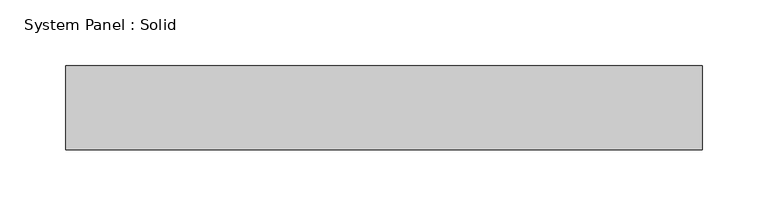
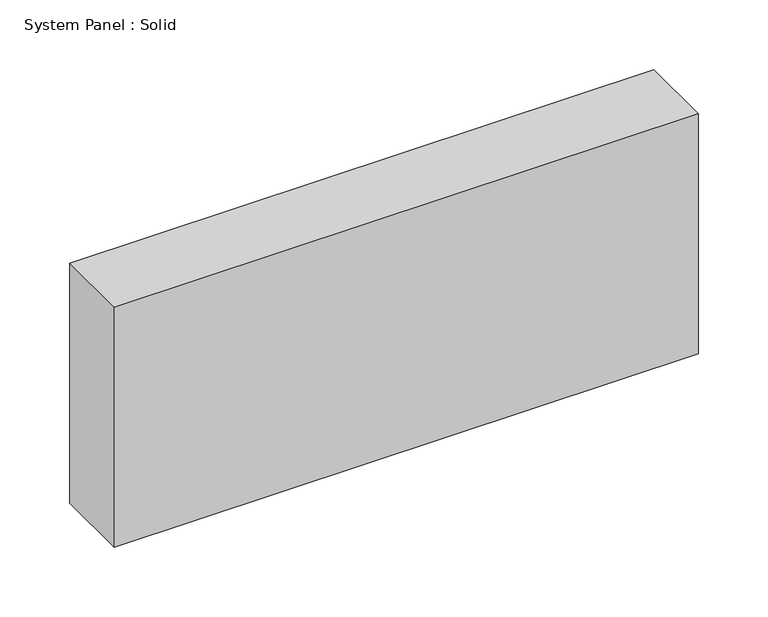
"""IFC4 building model written with IfcOpenShell, lengths in millimetres: plate geometry, System Panel : Solid."""

from ifc_helpers import new_model, si_unit, origin, origin_with_axes, place, context, project, spatial, polyline, outline, extrude, source, transform, mapped, element, save


def system_panel_solid_a8a40995(model_context):
    return source(origin(), model_context, "Body", "SweptSolid", [
        extrude(outline(polyline([(241.3, -19.05), (-241.3, -19.05), (-241.3, 44.45), (241.3, 44.45), (241.3, -19.05)])), origin_with_axes(), (0.0, 0.0, 1.0), 209.55),
    ])


if __name__ == "__main__":
    model = new_model("IFC4")
    model_context = context("Model", 3, world=origin())
    ifc_project = project(units=[si_unit("LENGTHUNIT", "METRE", prefix="MILLI")], contexts=[model_context])
    site = spatial("IfcSite", under=ifc_project)
    building = spatial("IfcBuilding", under=site)
    placement = place(None, origin())
    system_panel_solid_shape = system_panel_solid_a8a40995(model_context)
    element("IfcPlate", 1, ObjectType="System Panel : Solid", at=placement, inside=building, context=model_context, shape_type="MappedRepresentation", body=[
        mapped(system_panel_solid_shape, transform((0.0, 0.0, 0.0), x_axis=(1.0, 0.0, 0.0), y_axis=(0.0, 1.0, 0.0), z_axis=(0.0, 0.0, 1.0))),
    ])
    save(model, "model.ifc")

# Revit data of these elements
# Type "System Panel : Solid"
#   Construction Type Id = "MDOOR"
#   Analytic Construction = "Metal"
#   Visual Light Transmittance = 0
#   Solar Heat Gain Coefficient = 0
#   Heat Transfer Coefficient (U) = 0.651978 BTU/(h·ft²·°F)
#   Define Thermal Properties by = 1
# Element 1 (IfcPlate, "System Panel : Solid")
#   Materials on its faces: "Default"
# Materials
#   "Default": colour RGB 127 127 127, transparency 0, Cost = 0
